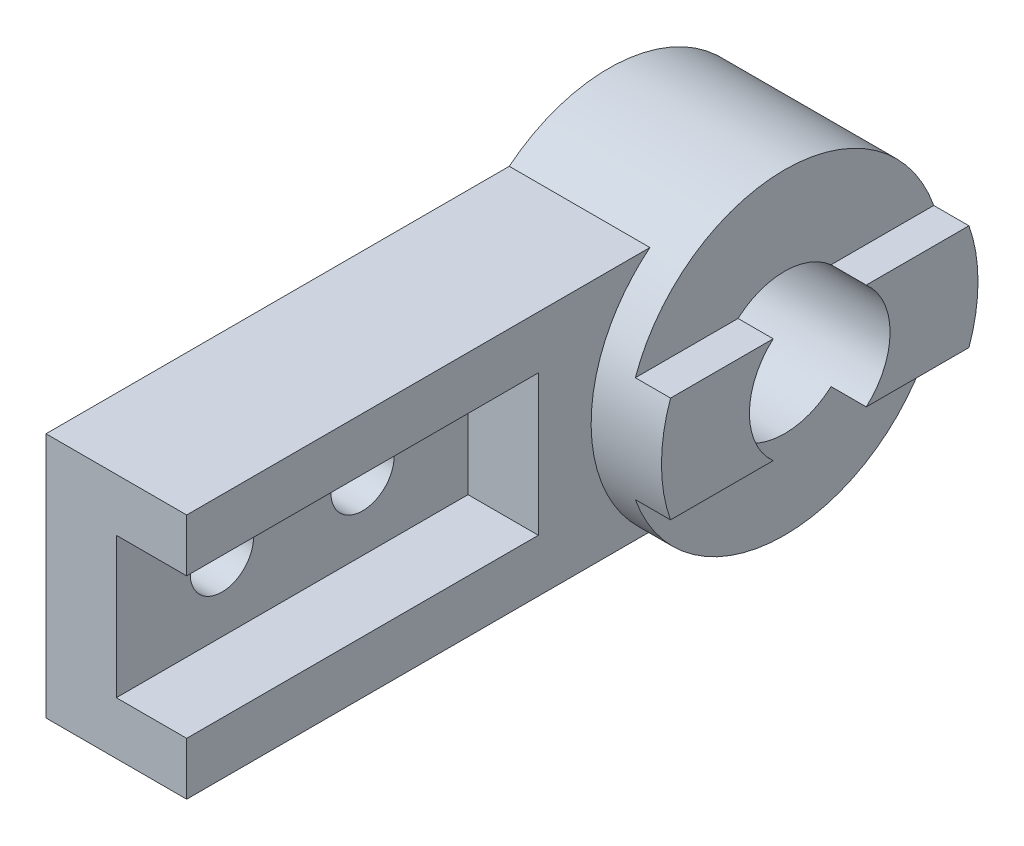
ISO-10303-21;
HEADER;
FILE_DESCRIPTION(('STEP AP214'),'2;1');
FILE_NAME('part.step','',(''),(''),'','','');
FILE_SCHEMA(('AUTOMOTIVE_DESIGN { 1 0 10303 214 1 1 1 1 }'));
ENDSEC;
DATA;
#1=APPLICATION_CONTEXT('core data for automotive mechanical design processes');
#2=APPLICATION_PROTOCOL_DEFINITION('international standard','automotive_design',2000,#1);
#3=PRODUCT_CONTEXT('',#1,'mechanical');
#4=PRODUCT('Part','Part','',(#3));
#5=PRODUCT_RELATED_PRODUCT_CATEGORY('part','',(#4));
#6=PRODUCT_DEFINITION_FORMATION('','',#4);
#7=PRODUCT_DEFINITION_CONTEXT('part definition',#1,'design');
#8=PRODUCT_DEFINITION('design','',#6,#7);
#9=PRODUCT_DEFINITION_SHAPE('','',#8);
#10=(LENGTH_UNIT() NAMED_UNIT(*) SI_UNIT(.MILLI.,.METRE.));
#11=(NAMED_UNIT(*) PLANE_ANGLE_UNIT() SI_UNIT($,.RADIAN.));
#12=(NAMED_UNIT(*) SI_UNIT($,.STERADIAN.) SOLID_ANGLE_UNIT());
#13=UNCERTAINTY_MEASURE_WITH_UNIT(LENGTH_MEASURE(1.E-05),#10,'distance_accuracy_value','');
#14=(GEOMETRIC_REPRESENTATION_CONTEXT(3) GLOBAL_UNCERTAINTY_ASSIGNED_CONTEXT((#13)) GLOBAL_UNIT_ASSIGNED_CONTEXT((#10,
#11,#12)) REPRESENTATION_CONTEXT('',''));
#15=CARTESIAN_POINT('',(0.,0.,0.));
#16=DIRECTION('',(0.,0.,1.));
#17=DIRECTION('',(1.,0.,0.));
#18=AXIS2_PLACEMENT_3D('',#15,#16,#17);
#19=CARTESIAN_POINT('',(20.,-17.5,80.));
#20=DIRECTION('',(-1.,0.,0.));
#21=DIRECTION('',(0.,-1.,0.));
#22=AXIS2_PLACEMENT_3D('',#19,#20,#21);
#23=PLANE('',#22);
#24=DIRECTION('',(0.,0.,1.));
#25=VECTOR('',#24,1.);
#26=CARTESIAN_POINT('',(20.,-10.,30.));
#27=LINE('',#26,#25);
#28=CARTESIAN_POINT('',(20.,-10.,30.));
#29=VERTEX_POINT('',#28);
#30=CARTESIAN_POINT('',(20.,-10.,80.));
#31=VERTEX_POINT('',#30);
#32=EDGE_CURVE('E171',#29,#31,#27,.T.);
#33=ORIENTED_EDGE('',*,*,#32,.T.);
#34=DIRECTION('',(0.,1.,0.));
#35=VECTOR('',#34,1.);
#36=CARTESIAN_POINT('',(20.,-17.5,80.));
#37=LINE('',#36,#35);
#38=CARTESIAN_POINT('',(20.,-17.5,80.));
#39=VERTEX_POINT('',#38);
#40=EDGE_CURVE('E189',#39,#31,#37,.T.);
#41=ORIENTED_EDGE('',*,*,#40,.F.);
#42=DIRECTION('',(0.,0.,-1.));
#43=VECTOR('',#42,1.);
#44=CARTESIAN_POINT('',(20.,-17.5,80.));
#45=LINE('',#44,#43);
#46=CARTESIAN_POINT('',(20.,-17.5,14.142135623731));
#47=VERTEX_POINT('',#46);
#48=EDGE_CURVE('E198',#39,#47,#45,.T.);
#49=ORIENTED_EDGE('',*,*,#48,.T.);
#50=CARTESIAN_POINT('',(20.,0.,0.));
#51=DIRECTION('',(-1.,0.,0.));
#52=DIRECTION('',(0.,-1.,0.));
#53=AXIS2_PLACEMENT_3D('',#50,#51,#52);
#54=CIRCLE('',#53,22.5);
#55=CARTESIAN_POINT('',(20.,17.5,14.1421356237309));
#56=VERTEX_POINT('',#55);
#57=EDGE_CURVE('E61',#47,#56,#54,.T.);
#58=ORIENTED_EDGE('',*,*,#57,.T.);
#59=DIRECTION('',(0.,0.,-1.));
#60=VECTOR('',#59,1.);
#61=CARTESIAN_POINT('',(20.,17.5,80.));
#62=LINE('',#61,#60);
#63=CARTESIAN_POINT('',(20.,17.5,80.));
#64=VERTEX_POINT('',#63);
#65=EDGE_CURVE('E196',#64,#56,#62,.T.);
#66=ORIENTED_EDGE('',*,*,#65,.F.);
#67=CARTESIAN_POINT('',(20.,10.,80.));
#68=VERTEX_POINT('',#67);
#69=EDGE_CURVE('E190',#68,#64,#37,.T.);
#70=ORIENTED_EDGE('',*,*,#69,.F.);
#71=DIRECTION('',(0.,0.,1.));
#72=VECTOR('',#71,1.);
#73=CARTESIAN_POINT('',(20.,10.,30.));
#74=LINE('',#73,#72);
#75=CARTESIAN_POINT('',(20.,10.,30.));
#76=VERTEX_POINT('',#75);
#77=EDGE_CURVE('E57',#76,#68,#74,.T.);
#78=ORIENTED_EDGE('',*,*,#77,.F.);
#79=DIRECTION('',(0.,1.,0.));
#80=VECTOR('',#79,1.);
#81=CARTESIAN_POINT('',(20.,-10.,30.));
#82=LINE('',#81,#80);
#83=EDGE_CURVE('E346',#29,#76,#82,.T.);
#84=ORIENTED_EDGE('',*,*,#83,.F.);
#85=EDGE_LOOP('',(#33,#41,#49,#58,#66,#70,#78,#84));
#86=FACE_BOUND('',#85,.T.);
#87=ADVANCED_FACE('F41',(#86),#23,.F.);
#88=CARTESIAN_POINT('',(0.,0.,80.));
#89=DIRECTION('',(0.,0.,1.));
#90=DIRECTION('',(1.,0.,0.));
#91=AXIS2_PLACEMENT_3D('',#88,#89,#90);
#92=PLANE('',#91);
#93=ORIENTED_EDGE('',*,*,#40,.T.);
#94=DIRECTION('',(-1.,0.,0.));
#95=VECTOR('',#94,1.);
#96=CARTESIAN_POINT('',(20.,-10.,80.));
#97=LINE('',#96,#95);
#98=CARTESIAN_POINT('',(10.,-10.,80.));
#99=VERTEX_POINT('',#98);
#100=EDGE_CURVE('E347',#31,#99,#97,.T.);
#101=ORIENTED_EDGE('',*,*,#100,.T.);
#102=DIRECTION('',(0.,1.,0.));
#103=VECTOR('',#102,1.);
#104=CARTESIAN_POINT('',(10.,-10.,80.));
#105=LINE('',#104,#103);
#106=CARTESIAN_POINT('',(10.,10.,80.));
#107=VERTEX_POINT('',#106);
#108=EDGE_CURVE('E176',#99,#107,#105,.T.);
#109=ORIENTED_EDGE('',*,*,#108,.T.);
#110=DIRECTION('',(-1.,0.,0.));
#111=VECTOR('',#110,1.);
#112=CARTESIAN_POINT('',(20.,10.,80.));
#113=LINE('',#112,#111);
#114=EDGE_CURVE('E175',#68,#107,#113,.T.);
#115=ORIENTED_EDGE('',*,*,#114,.F.);
#116=ORIENTED_EDGE('',*,*,#69,.T.);
#117=DIRECTION('',(-1.,0.,0.));
#118=VECTOR('',#117,1.);
#119=CARTESIAN_POINT('',(20.,17.5,80.));
#120=LINE('',#119,#118);
#121=CARTESIAN_POINT('',(0.,17.5,80.));
#122=VERTEX_POINT('',#121);
#123=EDGE_CURVE('E192',#64,#122,#120,.T.);
#124=ORIENTED_EDGE('',*,*,#123,.T.);
#125=DIRECTION('',(0.,-1.,0.));
#126=VECTOR('',#125,1.);
#127=CARTESIAN_POINT('',(0.,-17.5,80.));
#128=LINE('',#127,#126);
#129=CARTESIAN_POINT('',(0.,-17.5,80.));
#130=VERTEX_POINT('',#129);
#131=EDGE_CURVE('E180',#122,#130,#128,.T.);
#132=ORIENTED_EDGE('',*,*,#131,.T.);
#133=DIRECTION('',(1.,0.,0.));
#134=VECTOR('',#133,1.);
#135=CARTESIAN_POINT('',(20.,-17.5,80.));
#136=LINE('',#135,#134);
#137=EDGE_CURVE('E181',#130,#39,#136,.T.);
#138=ORIENTED_EDGE('',*,*,#137,.T.);
#139=EDGE_LOOP('',(#93,#101,#109,#115,#116,#124,#132,#138));
#140=FACE_BOUND('',#139,.T.);
#141=ADVANCED_FACE('F274',(#140),#92,.T.);
#142=CARTESIAN_POINT('',(30.,0.,0.));
#143=DIRECTION('',(-1.,0.,0.));
#144=DIRECTION('',(0.,0.,1.));
#145=AXIS2_PLACEMENT_3D('',#142,#143,#144);
#146=CYLINDRICAL_SURFACE('',#145,22.5);
#147=CARTESIAN_POINT('',(30.,0.,0.));
#148=DIRECTION('',(1.,0.,0.));
#149=DIRECTION('',(0.,0.,-1.));
#150=AXIS2_PLACEMENT_3D('',#147,#148,#149);
#151=CIRCLE('',#150,22.5);
#152=CARTESIAN_POINT('',(30.,-7.50000000000002,-21.2132034355964));
#153=VERTEX_POINT('',#152);
#154=CARTESIAN_POINT('',(30.,7.49999999999997,-21.2132034355964));
#155=VERTEX_POINT('',#154);
#156=EDGE_CURVE('E244',#153,#155,#151,.T.);
#157=ORIENTED_EDGE('',*,*,#156,.F.);
#158=DIRECTION('',(1.,0.,0.));
#159=VECTOR('',#158,1.);
#160=CARTESIAN_POINT('',(25.,-7.50000000000002,-21.2132034355964));
#161=LINE('',#160,#159);
#162=CARTESIAN_POINT('',(25.,-7.50000000000002,-21.2132034355964));
#163=VERTEX_POINT('',#162);
#164=EDGE_CURVE('E214',#163,#153,#161,.T.);
#165=ORIENTED_EDGE('',*,*,#164,.F.);
#166=CARTESIAN_POINT('',(25.,0.,0.));
#167=DIRECTION('',(1.,0.,0.));
#168=DIRECTION('',(0.,0.,-1.));
#169=AXIS2_PLACEMENT_3D('',#166,#167,#168);
#170=CIRCLE('',#169,22.5);
#171=CARTESIAN_POINT('',(25.,-7.50000000000002,21.2132034355964));
#172=VERTEX_POINT('',#171);
#173=EDGE_CURVE('E210',#172,#163,#170,.T.);
#174=ORIENTED_EDGE('',*,*,#173,.F.);
#175=DIRECTION('',(1.,0.,0.));
#176=VECTOR('',#175,1.);
#177=CARTESIAN_POINT('',(25.,-7.50000000000002,21.2132034355964));
#178=LINE('',#177,#176);
#179=CARTESIAN_POINT('',(30.,-7.50000000000002,21.2132034355964));
#180=VERTEX_POINT('',#179);
#181=EDGE_CURVE('E213',#172,#180,#178,.T.);
#182=ORIENTED_EDGE('',*,*,#181,.T.);
#183=CARTESIAN_POINT('',(30.,7.49999999999998,21.2132034355964));
#184=VERTEX_POINT('',#183);
#185=EDGE_CURVE('E241',#184,#180,#151,.T.);
#186=ORIENTED_EDGE('',*,*,#185,.F.);
#187=DIRECTION('',(1.,0.,0.));
#188=VECTOR('',#187,1.);
#189=CARTESIAN_POINT('',(25.,7.49999999999998,21.2132034355964));
#190=LINE('',#189,#188);
#191=CARTESIAN_POINT('',(25.,7.49999999999998,21.2132034355964));
#192=VERTEX_POINT('',#191);
#193=EDGE_CURVE('E230',#192,#184,#190,.T.);
#194=ORIENTED_EDGE('',*,*,#193,.F.);
#195=CARTESIAN_POINT('',(25.,0.,0.));
#196=DIRECTION('',(-1.,0.,0.));
#197=DIRECTION('',(0.,0.,1.));
#198=AXIS2_PLACEMENT_3D('',#195,#196,#197);
#199=CIRCLE('',#198,22.5);
#200=CARTESIAN_POINT('',(25.,7.49999999999997,-21.2132034355964));
#201=VERTEX_POINT('',#200);
#202=EDGE_CURVE('E221',#192,#201,#199,.T.);
#203=ORIENTED_EDGE('',*,*,#202,.T.);
#204=DIRECTION('',(1.,0.,0.));
#205=VECTOR('',#204,1.);
#206=CARTESIAN_POINT('',(25.,7.49999999999997,-21.2132034355964));
#207=LINE('',#206,#205);
#208=EDGE_CURVE('E228',#201,#155,#207,.T.);
#209=ORIENTED_EDGE('',*,*,#208,.T.);
#210=EDGE_LOOP('',(#157,#165,#174,#182,#186,#194,#203,#209));
#211=FACE_BOUND('',#210,.T.);
#212=DIRECTION('',(-1.,0.,0.));
#213=VECTOR('',#212,1.);
#214=CARTESIAN_POINT('',(30.,-17.5,14.142135623731));
#215=LINE('',#214,#213);
#216=CARTESIAN_POINT('',(0.,-17.5,14.142135623731));
#217=VERTEX_POINT('',#216);
#218=EDGE_CURVE('E11',#217,#47,#215,.F.);
#219=ORIENTED_EDGE('',*,*,#218,.F.);
#220=CARTESIAN_POINT('',(0.,0.,0.));
#221=DIRECTION('',(1.,0.,0.));
#222=DIRECTION('',(0.,0.,-1.));
#223=AXIS2_PLACEMENT_3D('',#220,#221,#222);
#224=CIRCLE('',#223,22.5);
#225=CARTESIAN_POINT('',(0.,17.5,14.1421356237309));
#226=VERTEX_POINT('',#225);
#227=EDGE_CURVE('E240',#217,#226,#224,.T.);
#228=ORIENTED_EDGE('',*,*,#227,.T.);
#229=DIRECTION('',(-1.,0.,0.));
#230=VECTOR('',#229,1.);
#231=CARTESIAN_POINT('',(30.,17.5,14.1421356237309));
#232=LINE('',#231,#230);
#233=EDGE_CURVE('E47',#56,#226,#232,.T.);
#234=ORIENTED_EDGE('',*,*,#233,.F.);
#235=ORIENTED_EDGE('',*,*,#57,.F.);
#236=EDGE_LOOP('',(#219,#228,#234,#235));
#237=FACE_BOUND('',#236,.T.);
#238=ADVANCED_FACE('F43',(#211,#237),#146,.T.);
#239=CARTESIAN_POINT('',(30.,0.,0.));
#240=DIRECTION('',(-1.,0.,0.));
#241=DIRECTION('',(0.,0.,1.));
#242=AXIS2_PLACEMENT_3D('',#239,#240,#241);
#243=CYLINDRICAL_SURFACE('',#242,10.);
#244=CARTESIAN_POINT('',(0.,0.,0.));
#245=DIRECTION('',(1.,0.,0.));
#246=DIRECTION('',(0.,0.,-1.));
#247=AXIS2_PLACEMENT_3D('',#244,#245,#246);
#248=CIRCLE('',#247,10.);
#249=CARTESIAN_POINT('',(0.,0.,-10.));
#250=VERTEX_POINT('',#249);
#251=EDGE_CURVE('E233',#250,#250,#248,.T.);
#252=ORIENTED_EDGE('',*,*,#251,.F.);
#253=EDGE_LOOP('',(#252));
#254=FACE_BOUND('',#253,.T.);
#255=DIRECTION('',(-1.,0.,0.));
#256=VECTOR('',#255,1.);
#257=CARTESIAN_POINT('',(30.,-7.50000000000002,-6.61437827766145));
#258=LINE('',#257,#256);
#259=CARTESIAN_POINT('',(30.,-7.50000000000002,-6.61437827766145));
#260=VERTEX_POINT('',#259);
#261=CARTESIAN_POINT('',(25.,-7.50000000000002,-6.61437827766145));
#262=VERTEX_POINT('',#261);
#263=EDGE_CURVE('E256',#260,#262,#258,.T.);
#264=ORIENTED_EDGE('',*,*,#263,.F.);
#265=CARTESIAN_POINT('',(30.,0.,0.));
#266=DIRECTION('',(1.,0.,0.));
#267=DIRECTION('',(0.,0.,-1.));
#268=AXIS2_PLACEMENT_3D('',#265,#266,#267);
#269=CIRCLE('',#268,10.);
#270=CARTESIAN_POINT('',(30.,7.49999999999998,-6.6143782776615));
#271=VERTEX_POINT('',#270);
#272=EDGE_CURVE('E238',#260,#271,#269,.T.);
#273=ORIENTED_EDGE('',*,*,#272,.T.);
#274=DIRECTION('',(-1.,0.,0.));
#275=VECTOR('',#274,1.);
#276=CARTESIAN_POINT('',(30.,7.49999999999998,-6.6143782776615));
#277=LINE('',#276,#275);
#278=CARTESIAN_POINT('',(25.,7.49999999999998,-6.6143782776615));
#279=VERTEX_POINT('',#278);
#280=EDGE_CURVE('E247',#279,#271,#277,.F.);
#281=ORIENTED_EDGE('',*,*,#280,.F.);
#282=CARTESIAN_POINT('',(25.,0.,0.));
#283=DIRECTION('',(-1.,0.,0.));
#284=DIRECTION('',(0.,0.,1.));
#285=AXIS2_PLACEMENT_3D('',#282,#283,#284);
#286=CIRCLE('',#285,10.);
#287=CARTESIAN_POINT('',(25.,7.49999999999998,6.6143782776615));
#288=VERTEX_POINT('',#287);
#289=EDGE_CURVE('E242',#288,#279,#286,.T.);
#290=ORIENTED_EDGE('',*,*,#289,.F.);
#291=DIRECTION('',(-1.,0.,0.));
#292=VECTOR('',#291,1.);
#293=CARTESIAN_POINT('',(30.,7.49999999999998,6.6143782776615));
#294=LINE('',#293,#292);
#295=CARTESIAN_POINT('',(30.,7.49999999999998,6.6143782776615));
#296=VERTEX_POINT('',#295);
#297=EDGE_CURVE('E252',#296,#288,#294,.T.);
#298=ORIENTED_EDGE('',*,*,#297,.F.);
#299=CARTESIAN_POINT('',(30.,-7.50000000000002,6.61437827766145));
#300=VERTEX_POINT('',#299);
#301=EDGE_CURVE('E234',#296,#300,#269,.T.);
#302=ORIENTED_EDGE('',*,*,#301,.T.);
#303=DIRECTION('',(-1.,0.,0.));
#304=VECTOR('',#303,1.);
#305=CARTESIAN_POINT('',(30.,-7.50000000000002,6.61437827766145));
#306=LINE('',#305,#304);
#307=CARTESIAN_POINT('',(25.,-7.50000000000002,6.61437827766145));
#308=VERTEX_POINT('',#307);
#309=EDGE_CURVE('E260',#308,#300,#306,.F.);
#310=ORIENTED_EDGE('',*,*,#309,.F.);
#311=CARTESIAN_POINT('',(25.,0.,0.));
#312=DIRECTION('',(1.,0.,0.));
#313=DIRECTION('',(0.,0.,-1.));
#314=AXIS2_PLACEMENT_3D('',#311,#312,#313);
#315=CIRCLE('',#314,10.);
#316=EDGE_CURVE('E251',#308,#262,#315,.T.);
#317=ORIENTED_EDGE('',*,*,#316,.T.);
#318=EDGE_LOOP('',(#264,#273,#281,#290,#298,#302,#310,#317));
#319=FACE_BOUND('',#318,.T.);
#320=ADVANCED_FACE('F285',(#254,#319),#243,.F.);
#321=CARTESIAN_POINT('',(30.,0.,0.));
#322=DIRECTION('',(1.,0.,0.));
#323=DIRECTION('',(0.,0.,-1.));
#324=AXIS2_PLACEMENT_3D('',#321,#322,#323);
#325=PLANE('',#324);
#326=DIRECTION('',(0.,0.,1.));
#327=VECTOR('',#326,1.);
#328=CARTESIAN_POINT('',(30.,-7.50000000000002,21.2132034355964));
#329=LINE('',#328,#327);
#330=EDGE_CURVE('E208',#153,#260,#329,.T.);
#331=ORIENTED_EDGE('',*,*,#330,.F.);
#332=ORIENTED_EDGE('',*,*,#156,.T.);
#333=DIRECTION('',(0.,0.,-1.));
#334=VECTOR('',#333,1.);
#335=CARTESIAN_POINT('',(30.,7.49999999999998,21.2132034355964));
#336=LINE('',#335,#334);
#337=EDGE_CURVE('E217',#271,#155,#336,.T.);
#338=ORIENTED_EDGE('',*,*,#337,.F.);
#339=ORIENTED_EDGE('',*,*,#272,.F.);
#340=EDGE_LOOP('',(#331,#332,#338,#339));
#341=FACE_BOUND('',#340,.T.);
#342=ADVANCED_FACE('F288',(#341),#325,.T.);
#343=EDGE_CURVE('E207',#300,#180,#329,.T.);
#344=ORIENTED_EDGE('',*,*,#343,.F.);
#345=ORIENTED_EDGE('',*,*,#301,.F.);
#346=EDGE_CURVE('E227',#184,#296,#336,.T.);
#347=ORIENTED_EDGE('',*,*,#346,.F.);
#348=ORIENTED_EDGE('',*,*,#185,.T.);
#349=EDGE_LOOP('',(#344,#345,#347,#348));
#350=FACE_BOUND('',#349,.T.);
#351=ADVANCED_FACE('F316',(#350),#325,.T.);
#352=CARTESIAN_POINT('',(0.,0.,0.));
#353=DIRECTION('',(1.,0.,0.));
#354=DIRECTION('',(0.,0.,-1.));
#355=AXIS2_PLACEMENT_3D('',#352,#353,#354);
#356=PLANE('',#355);
#357=CARTESIAN_POINT('',(0.,0.,65.));
#358=DIRECTION('',(1.,0.,0.));
#359=DIRECTION('',(0.,0.,-1.));
#360=AXIS2_PLACEMENT_3D('',#357,#358,#359);
#361=CIRCLE('',#360,4.5);
#362=CARTESIAN_POINT('',(0.,0.,60.5));
#363=VERTEX_POINT('',#362);
#364=EDGE_CURVE('E335',#363,#363,#361,.T.);
#365=ORIENTED_EDGE('',*,*,#364,.T.);
#366=EDGE_LOOP('',(#365));
#367=FACE_BOUND('',#366,.T.);
#368=CARTESIAN_POINT('',(0.,0.,45.));
#369=DIRECTION('',(1.,0.,0.));
#370=DIRECTION('',(0.,0.,-1.));
#371=AXIS2_PLACEMENT_3D('',#368,#369,#370);
#372=CIRCLE('',#371,4.5);
#373=CARTESIAN_POINT('',(0.,0.,40.5));
#374=VERTEX_POINT('',#373);
#375=EDGE_CURVE('E337',#374,#374,#372,.T.);
#376=ORIENTED_EDGE('',*,*,#375,.T.);
#377=EDGE_LOOP('',(#376));
#378=FACE_BOUND('',#377,.T.);
#379=ORIENTED_EDGE('',*,*,#227,.F.);
#380=DIRECTION('',(0.,0.,-1.));
#381=VECTOR('',#380,1.);
#382=CARTESIAN_POINT('',(0.,-17.5,80.));
#383=LINE('',#382,#381);
#384=EDGE_CURVE('E201',#130,#217,#383,.T.);
#385=ORIENTED_EDGE('',*,*,#384,.F.);
#386=ORIENTED_EDGE('',*,*,#131,.F.);
#387=DIRECTION('',(0.,0.,-1.));
#388=VECTOR('',#387,1.);
#389=CARTESIAN_POINT('',(0.,17.5,80.));
#390=LINE('',#389,#388);
#391=EDGE_CURVE('E194',#122,#226,#390,.T.);
#392=ORIENTED_EDGE('',*,*,#391,.T.);
#393=EDGE_LOOP('',(#379,#385,#386,#392));
#394=FACE_BOUND('',#393,.T.);
#395=ORIENTED_EDGE('',*,*,#251,.T.);
#396=EDGE_LOOP('',(#395));
#397=FACE_BOUND('',#396,.T.);
#398=ADVANCED_FACE('F267',(#367,#378,#394,#397),#356,.F.);
#399=CARTESIAN_POINT('',(25.,7.49999999999998,21.2132034355964));
#400=DIRECTION('',(0.,-1.,0.));
#401=DIRECTION('',(0.,0.,-1.));
#402=AXIS2_PLACEMENT_3D('',#399,#400,#401);
#403=PLANE('',#402);
#404=ORIENTED_EDGE('',*,*,#297,.T.);
#405=DIRECTION('',(0.,0.,-1.));
#406=VECTOR('',#405,1.);
#407=CARTESIAN_POINT('',(25.,7.49999999999998,21.2132034355964));
#408=LINE('',#407,#406);
#409=EDGE_CURVE('E219',#192,#288,#408,.T.);
#410=ORIENTED_EDGE('',*,*,#409,.F.);
#411=ORIENTED_EDGE('',*,*,#193,.T.);
#412=ORIENTED_EDGE('',*,*,#346,.T.);
#413=EDGE_LOOP('',(#404,#410,#411,#412));
#414=FACE_BOUND('',#413,.T.);
#415=ADVANCED_FACE('F317',(#414),#403,.F.);
#416=ORIENTED_EDGE('',*,*,#280,.T.);
#417=ORIENTED_EDGE('',*,*,#337,.T.);
#418=ORIENTED_EDGE('',*,*,#208,.F.);
#419=EDGE_CURVE('E225',#279,#201,#408,.T.);
#420=ORIENTED_EDGE('',*,*,#419,.F.);
#421=EDGE_LOOP('',(#416,#417,#418,#420));
#422=FACE_BOUND('',#421,.T.);
#423=ADVANCED_FACE('F312',(#422),#403,.F.);
#424=CARTESIAN_POINT('',(25.,0.,0.));
#425=DIRECTION('',(-1.,0.,0.));
#426=DIRECTION('',(0.,0.,1.));
#427=AXIS2_PLACEMENT_3D('',#424,#425,#426);
#428=PLANE('',#427);
#429=ORIENTED_EDGE('',*,*,#289,.T.);
#430=ORIENTED_EDGE('',*,*,#419,.T.);
#431=ORIENTED_EDGE('',*,*,#202,.F.);
#432=ORIENTED_EDGE('',*,*,#409,.T.);
#433=EDGE_LOOP('',(#429,#430,#431,#432));
#434=FACE_BOUND('',#433,.T.);
#435=ADVANCED_FACE('F309',(#434),#428,.F.);
#436=CARTESIAN_POINT('',(25.,-7.50000000000002,21.2132034355964));
#437=DIRECTION('',(0.,1.,0.));
#438=DIRECTION('',(0.,0.,1.));
#439=AXIS2_PLACEMENT_3D('',#436,#437,#438);
#440=PLANE('',#439);
#441=ORIENTED_EDGE('',*,*,#263,.T.);
#442=DIRECTION('',(0.,0.,1.));
#443=VECTOR('',#442,1.);
#444=CARTESIAN_POINT('',(25.,-7.50000000000002,21.2132034355964));
#445=LINE('',#444,#443);
#446=EDGE_CURVE('E212',#163,#262,#445,.T.);
#447=ORIENTED_EDGE('',*,*,#446,.F.);
#448=ORIENTED_EDGE('',*,*,#164,.T.);
#449=ORIENTED_EDGE('',*,*,#330,.T.);
#450=EDGE_LOOP('',(#441,#447,#448,#449));
#451=FACE_BOUND('',#450,.T.);
#452=ADVANCED_FACE('F308',(#451),#440,.F.);
#453=ORIENTED_EDGE('',*,*,#309,.T.);
#454=ORIENTED_EDGE('',*,*,#343,.T.);
#455=ORIENTED_EDGE('',*,*,#181,.F.);
#456=EDGE_CURVE('E209',#308,#172,#445,.T.);
#457=ORIENTED_EDGE('',*,*,#456,.F.);
#458=EDGE_LOOP('',(#453,#454,#455,#457));
#459=FACE_BOUND('',#458,.T.);
#460=ADVANCED_FACE('F302',(#459),#440,.F.);
#461=CARTESIAN_POINT('',(25.,0.,0.));
#462=DIRECTION('',(1.,0.,0.));
#463=DIRECTION('',(0.,0.,-1.));
#464=AXIS2_PLACEMENT_3D('',#461,#462,#463);
#465=PLANE('',#464);
#466=ORIENTED_EDGE('',*,*,#456,.T.);
#467=ORIENTED_EDGE('',*,*,#173,.T.);
#468=ORIENTED_EDGE('',*,*,#446,.T.);
#469=ORIENTED_EDGE('',*,*,#316,.F.);
#470=EDGE_LOOP('',(#466,#467,#468,#469));
#471=FACE_BOUND('',#470,.T.);
#472=ADVANCED_FACE('F305',(#471),#465,.T.);
#473=CARTESIAN_POINT('',(20.,-17.5,80.));
#474=DIRECTION('',(0.,1.,0.));
#475=DIRECTION('',(-1.,0.,0.));
#476=AXIS2_PLACEMENT_3D('',#473,#474,#475);
#477=PLANE('',#476);
#478=ORIENTED_EDGE('',*,*,#384,.T.);
#479=ORIENTED_EDGE('',*,*,#218,.T.);
#480=ORIENTED_EDGE('',*,*,#48,.F.);
#481=ORIENTED_EDGE('',*,*,#137,.F.);
#482=EDGE_LOOP('',(#478,#479,#480,#481));
#483=FACE_BOUND('',#482,.T.);
#484=ADVANCED_FACE('F278',(#483),#477,.F.);
#485=CARTESIAN_POINT('',(20.,17.5,80.));
#486=DIRECTION('',(0.,-1.,0.));
#487=DIRECTION('',(1.,0.,0.));
#488=AXIS2_PLACEMENT_3D('',#485,#486,#487);
#489=PLANE('',#488);
#490=ORIENTED_EDGE('',*,*,#65,.T.);
#491=ORIENTED_EDGE('',*,*,#233,.T.);
#492=ORIENTED_EDGE('',*,*,#391,.F.);
#493=ORIENTED_EDGE('',*,*,#123,.F.);
#494=EDGE_LOOP('',(#490,#491,#492,#493));
#495=FACE_BOUND('',#494,.T.);
#496=ADVANCED_FACE('F263',(#495),#489,.F.);
#497=CARTESIAN_POINT('',(20.,-10.,30.));
#498=DIRECTION('',(0.,1.,0.));
#499=DIRECTION('',(0.,0.,1.));
#500=AXIS2_PLACEMENT_3D('',#497,#498,#499);
#501=PLANE('',#500);
#502=ORIENTED_EDGE('',*,*,#100,.F.);
#503=ORIENTED_EDGE('',*,*,#32,.F.);
#504=DIRECTION('',(-1.,0.,0.));
#505=VECTOR('',#504,1.);
#506=CARTESIAN_POINT('',(20.,-10.,30.));
#507=LINE('',#506,#505);
#508=CARTESIAN_POINT('',(10.,-10.,30.));
#509=VERTEX_POINT('',#508);
#510=EDGE_CURVE('E160',#29,#509,#507,.T.);
#511=ORIENTED_EDGE('',*,*,#510,.T.);
#512=DIRECTION('',(0.,0.,1.));
#513=VECTOR('',#512,1.);
#514=CARTESIAN_POINT('',(10.,-10.,30.));
#515=LINE('',#514,#513);
#516=EDGE_CURVE('E166',#509,#99,#515,.T.);
#517=ORIENTED_EDGE('',*,*,#516,.T.);
#518=EDGE_LOOP('',(#502,#503,#511,#517));
#519=FACE_BOUND('',#518,.T.);
#520=ADVANCED_FACE('F170',(#519),#501,.T.);
#521=CARTESIAN_POINT('',(10.,-10.,30.));
#522=DIRECTION('',(1.,0.,0.));
#523=DIRECTION('',(0.,0.,-1.));
#524=AXIS2_PLACEMENT_3D('',#521,#522,#523);
#525=PLANE('',#524);
#526=CARTESIAN_POINT('',(10.,0.,65.));
#527=DIRECTION('',(1.,0.,0.));
#528=DIRECTION('',(0.,0.,-1.));
#529=AXIS2_PLACEMENT_3D('',#526,#527,#528);
#530=CIRCLE('',#529,4.5);
#531=CARTESIAN_POINT('',(10.,0.,60.5));
#532=VERTEX_POINT('',#531);
#533=EDGE_CURVE('E342',#532,#532,#530,.T.);
#534=ORIENTED_EDGE('',*,*,#533,.F.);
#535=EDGE_LOOP('',(#534));
#536=FACE_BOUND('',#535,.T.);
#537=CARTESIAN_POINT('',(10.,0.,45.));
#538=DIRECTION('',(1.,0.,0.));
#539=DIRECTION('',(0.,0.,-1.));
#540=AXIS2_PLACEMENT_3D('',#537,#538,#539);
#541=CIRCLE('',#540,4.5);
#542=CARTESIAN_POINT('',(10.,0.,40.5));
#543=VERTEX_POINT('',#542);
#544=EDGE_CURVE('E336',#543,#543,#541,.T.);
#545=ORIENTED_EDGE('',*,*,#544,.F.);
#546=EDGE_LOOP('',(#545));
#547=FACE_BOUND('',#546,.T.);
#548=ORIENTED_EDGE('',*,*,#108,.F.);
#549=ORIENTED_EDGE('',*,*,#516,.F.);
#550=DIRECTION('',(0.,1.,0.));
#551=VECTOR('',#550,1.);
#552=CARTESIAN_POINT('',(10.,-10.,30.));
#553=LINE('',#552,#551);
#554=CARTESIAN_POINT('',(10.,10.,30.));
#555=VERTEX_POINT('',#554);
#556=EDGE_CURVE('E153',#509,#555,#553,.T.);
#557=ORIENTED_EDGE('',*,*,#556,.T.);
#558=DIRECTION('',(0.,0.,1.));
#559=VECTOR('',#558,1.);
#560=CARTESIAN_POINT('',(10.,10.,30.));
#561=LINE('',#560,#559);
#562=EDGE_CURVE('E178',#555,#107,#561,.T.);
#563=ORIENTED_EDGE('',*,*,#562,.T.);
#564=EDGE_LOOP('',(#548,#549,#557,#563));
#565=FACE_BOUND('',#564,.T.);
#566=ADVANCED_FACE('F172',(#536,#547,#565),#525,.T.);
#567=CARTESIAN_POINT('',(20.,10.,30.));
#568=DIRECTION('',(0.,1.,0.));
#569=DIRECTION('',(0.,0.,1.));
#570=AXIS2_PLACEMENT_3D('',#567,#568,#569);
#571=PLANE('',#570);
#572=ORIENTED_EDGE('',*,*,#114,.T.);
#573=ORIENTED_EDGE('',*,*,#562,.F.);
#574=DIRECTION('',(-1.,0.,0.));
#575=VECTOR('',#574,1.);
#576=CARTESIAN_POINT('',(20.,10.,30.));
#577=LINE('',#576,#575);
#578=EDGE_CURVE('E157',#76,#555,#577,.T.);
#579=ORIENTED_EDGE('',*,*,#578,.F.);
#580=ORIENTED_EDGE('',*,*,#77,.T.);
#581=EDGE_LOOP('',(#572,#573,#579,#580));
#582=FACE_BOUND('',#581,.T.);
#583=ADVANCED_FACE('F351',(#582),#571,.F.);
#584=CARTESIAN_POINT('',(0.,0.,30.));
#585=DIRECTION('',(0.,0.,-1.));
#586=DIRECTION('',(-1.,0.,0.));
#587=AXIS2_PLACEMENT_3D('',#584,#585,#586);
#588=PLANE('',#587);
#589=ORIENTED_EDGE('',*,*,#510,.F.);
#590=ORIENTED_EDGE('',*,*,#83,.T.);
#591=ORIENTED_EDGE('',*,*,#578,.T.);
#592=ORIENTED_EDGE('',*,*,#556,.F.);
#593=EDGE_LOOP('',(#589,#590,#591,#592));
#594=FACE_BOUND('',#593,.T.);
#595=ADVANCED_FACE('F159',(#594),#588,.F.);
#596=CARTESIAN_POINT('',(0.,0.,45.));
#597=DIRECTION('',(1.,0.,0.));
#598=DIRECTION('',(0.,0.,-1.));
#599=AXIS2_PLACEMENT_3D('',#596,#597,#598);
#600=CYLINDRICAL_SURFACE('',#599,4.5);
#601=ORIENTED_EDGE('',*,*,#375,.F.);
#602=EDGE_LOOP('',(#601));
#603=FACE_BOUND('',#602,.T.);
#604=ORIENTED_EDGE('',*,*,#544,.T.);
#605=EDGE_LOOP('',(#604));
#606=FACE_BOUND('',#605,.T.);
#607=ADVANCED_FACE('F356',(#603,#606),#600,.F.);
#608=CARTESIAN_POINT('',(0.,0.,65.));
#609=DIRECTION('',(1.,0.,0.));
#610=DIRECTION('',(0.,0.,-1.));
#611=AXIS2_PLACEMENT_3D('',#608,#609,#610);
#612=CYLINDRICAL_SURFACE('',#611,4.5);
#613=ORIENTED_EDGE('',*,*,#364,.F.);
#614=EDGE_LOOP('',(#613));
#615=FACE_BOUND('',#614,.T.);
#616=ORIENTED_EDGE('',*,*,#533,.T.);
#617=EDGE_LOOP('',(#616));
#618=FACE_BOUND('',#617,.T.);
#619=ADVANCED_FACE('F416',(#615,#618),#612,.F.);
#620=CLOSED_SHELL('',(#87,#141,#238,#320,#342,#351,#398,#415,#423,#435,#452,#460,#472,#484,#496,
#520,#566,#583,#595,#607,#619));
#621=MANIFOLD_SOLID_BREP('B2',#620);
#622=ADVANCED_BREP_SHAPE_REPRESENTATION('',(#18,#621),#14);
#623=SHAPE_DEFINITION_REPRESENTATION(#9,#622);
ENDSEC;
END-ISO-10303-21;
